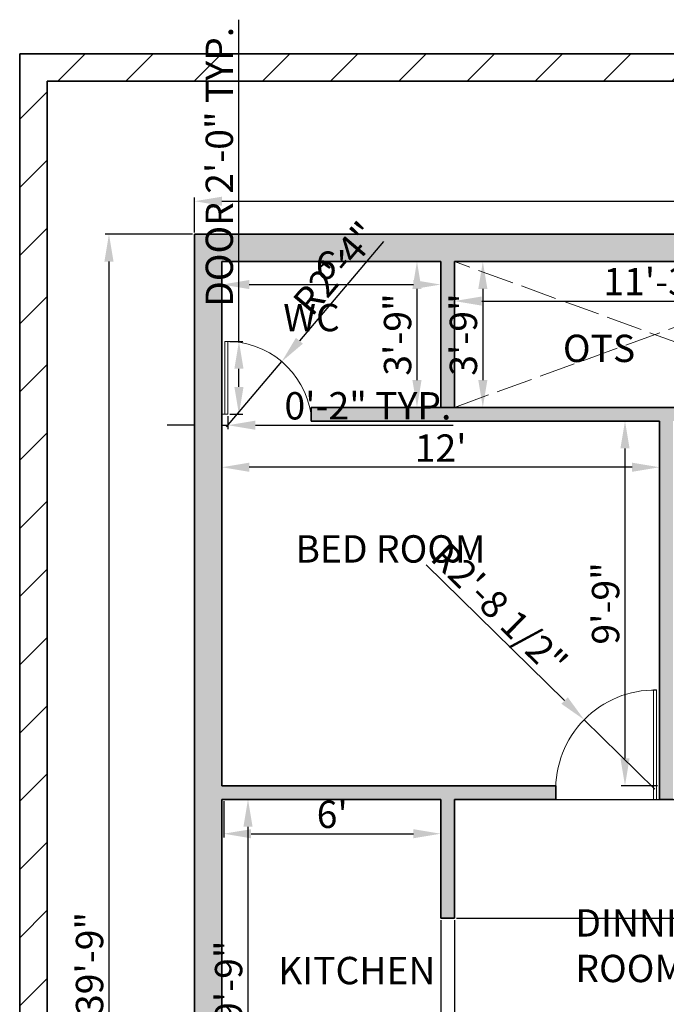
# Model space of a CAD drawing. Units: inches. Extents: x 1130698 to 1131150, y 432269 to 432875.
# Tile 2 of 3: x 1130698 to 1130911, y 432551 to 432875. Entities that reach past the tile are written whole.
import ezdxf

# ---------------------------------------------------------------- set-up
doc = ezdxf.new("R2010")
doc.units = ezdxf.units.IN
doc.linetypes.add('ACAD_ISO02W100', pattern=[15, 12, -3])
for name, color, linetype, lineweight in [('A-ANNO-DIMS', 2, 'Continuous', 18), ('A-ANNO-TTLB', 7, 'Continuous', 35), ('A-AREA-IDEN', 7, 'Continuous', 25), ('A-DOOR', 4, 'Continuous', 18), ('A-ROOF-OVHD', 8, 'ACAD_ISO02W100', 13), ('A-WALL', 7, 'Continuous', 35)]:
    doc.layers.add(name, color=color, linetype=linetype, lineweight=lineweight)
doc.layers.add('A-ANNO-TTLB-PATT', color=251, linetype='Continuous', lineweight=13, true_color=0x636466)
doc.layers.add('A-WALL-PATT', color=251, linetype='Continuous', lineweight=13, true_color=0x636466)
doc.styles.get("Standard").update_dxf_attribs({"font": 'arial.ttf'})
doc.dimstyles.new('ISO-25', dxfattribs={"dimtxt": 9, "dimasz": 9, "dimexe": 1.25, "dimexo": 0.625, "dimtad": 1, "dimdec": 1, "dimrnd": 9, "dimlunit": 3, "dimtxsty": 'Standard', "dimcen": 2.5, "dimadec": 0, "dimazin": 0, "dimtfac": 1, "dimtdec": 1, "dimtmove": 0, "dimatfit": 3, "dimfxl": 1, "dimarcsym": 0})

# ---------------------------------------------------------------- blocks, each defined once
blk = doc.blocks.new('*D1')
at = {"layer": 'A-ANNO-DIMS', "color": 0, "lineweight": -2, "transparency": 16777216}
for p, q in [((1130764.75, 432794.98), (1130764.75, 432786.8)), ((1130836.75, 432794.98), (1130836.75, 432786.8)), ((1130773.75, 432788.05), (1130827.75, 432788.05))]:
    blk.add_line(p, q, dxfattribs=at)
at = {"layer": 'A-ANNO-DIMS', "color": 0, "transparency": 16777216}
for points in [[(1130773.75, 432789.55), (1130773.75, 432786.55), (1130764.75, 432788.05)], [(1130827.75, 432789.55), (1130827.75, 432786.55), (1130836.75, 432788.05)]]:
    blk.add_solid(points, dxfattribs=at)
at = {"layer": 'Defpoints', "color": 0, "transparency": 16777216}
for p in [(1130764.75, 432795.61), (1130836.75, 432795.61), (1130836.75, 432788.05)]:
    blk.add_point(p, dxfattribs=at)
at = {"layer": 'A-ANNO-DIMS', "color": 0, "transparency": 16777216, "insert": (1130800.75, 432793.27), "char_height": 9, "attachment_point": 5}
blk.add_mtext("6'", dxfattribs=at)
blk = doc.blocks.new('*D2')
at = {"layer": 'A-ANNO-DIMS', "color": 0, "lineweight": -2, "transparency": 16777216}
for p, q in [((1130836.12, 432795.61), (1130827.69, 432795.61)), ((1130828.94, 432786.61), (1130828.94, 432756.61)), ((1130836.12, 432747.61), (1130827.69, 432747.61))]:
    blk.add_line(p, q, dxfattribs=at)
at = {"layer": 'A-ANNO-DIMS', "color": 0, "transparency": 16777216}
for points in [[(1130827.44, 432786.61), (1130830.44, 432786.61), (1130828.94, 432795.61)], [(1130827.44, 432756.61), (1130830.44, 432756.61), (1130828.94, 432747.61)]]:
    blk.add_solid(points, dxfattribs=at)
at = {"layer": 'Defpoints', "color": 0, "transparency": 16777216}
for p in [(1130836.75, 432795.61), (1130828.94, 432747.61), (1130836.75, 432747.61)]:
    blk.add_point(p, dxfattribs=at)
at = {"layer": 'A-ANNO-DIMS', "color": 0, "transparency": 16777216, "insert": (1130823.72, 432771.61), "char_height": 9, "attachment_point": 5, "rotation": 90}
blk.add_mtext('3\'-9"', dxfattribs=at)
blk = doc.blocks.new('*D3')
at = {"layer": 'A-ANNO-DIMS', "color": 0, "lineweight": -2, "transparency": 16777216}
for p, q in [((1130841.25, 432794.98), (1130841.25, 432781.37)), ((1130973.25, 432794.98), (1130973.25, 432781.37)), ((1130850.25, 432782.62), (1130964.25, 432782.62))]:
    blk.add_line(p, q, dxfattribs=at)
at = {"layer": 'A-ANNO-DIMS', "color": 0, "transparency": 16777216}
for points in [[(1130850.25, 432784.12), (1130850.25, 432781.12), (1130841.25, 432782.62)], [(1130964.25, 432784.12), (1130964.25, 432781.12), (1130973.25, 432782.62)]]:
    blk.add_solid(points, dxfattribs=at)
at = {"layer": 'Defpoints', "color": 0, "transparency": 16777216}
for p in [(1130841.25, 432795.61), (1130973.25, 432795.61), (1130973.25, 432782.62)]:
    blk.add_point(p, dxfattribs=at)
at = {"layer": 'A-ANNO-DIMS', "color": 0, "transparency": 16777216, "insert": (1130907.25, 432787.85), "char_height": 9, "attachment_point": 5}
blk.add_mtext('11\'-3"', dxfattribs=at)
blk = doc.blocks.new('*D4')
at = {"layer": 'A-ANNO-DIMS', "color": 0, "lineweight": -2, "transparency": 16777216}
for p, q in [((1130841.87, 432795.61), (1130851.87, 432795.61)), ((1130850.62, 432786.61), (1130850.62, 432756.61)), ((1130841.87, 432747.61), (1130851.87, 432747.61))]:
    blk.add_line(p, q, dxfattribs=at)
at = {"layer": 'A-ANNO-DIMS', "color": 0, "transparency": 16777216}
for points in [[(1130849.12, 432786.61), (1130852.12, 432786.61), (1130850.62, 432795.61)], [(1130849.12, 432756.61), (1130852.12, 432756.61), (1130850.62, 432747.61)]]:
    blk.add_solid(points, dxfattribs=at)
at = {"layer": 'Defpoints', "color": 0, "transparency": 16777216}
for p in [(1130841.25, 432795.61), (1130841.25, 432747.61), (1130850.62, 432747.61)]:
    blk.add_point(p, dxfattribs=at)
at = {"layer": 'A-ANNO-DIMS', "color": 0, "transparency": 16777216, "insert": (1130845.39, 432771.61), "char_height": 9, "attachment_point": 5, "rotation": 90}
blk.add_mtext('3\'-9"', dxfattribs=at)
blk = doc.blocks.new('*D7')
at = {"layer": 'A-ANNO-DIMS', "color": 0, "lineweight": -2, "transparency": 16777216}
for p, q in [((1130908.75, 432742.48), (1130908.75, 432726.67)), ((1130764.75, 432740.23), (1130764.75, 432726.67)), ((1130899.75, 432727.92), (1130773.75, 432727.92))]:
    blk.add_line(p, q, dxfattribs=at)
at = {"layer": 'A-ANNO-DIMS', "color": 0, "transparency": 16777216}
for points in [[(1130773.75, 432729.42), (1130773.75, 432726.42), (1130764.75, 432727.92)], [(1130899.75, 432729.42), (1130899.75, 432726.42), (1130908.75, 432727.92)]]:
    blk.add_solid(points, dxfattribs=at)
at = {"layer": 'Defpoints', "color": 0, "transparency": 16777216}
for p in [(1130908.75, 432743.11), (1130764.75, 432740.86), (1130764.75, 432727.92)]:
    blk.add_point(p, dxfattribs=at)
at = {"layer": 'A-ANNO-DIMS', "color": 0, "transparency": 16777216, "insert": (1130836.75, 432733.06), "char_height": 9, "attachment_point": 5}
blk.add_mtext("12'", dxfattribs=at)
blk = doc.blocks.new('*D8')
at = {"layer": 'A-ANNO-DIMS', "color": 0, "lineweight": -2, "transparency": 16777216}
for p, q in [((1130908.12, 432743.11), (1130896.15, 432743.11)), ((1130897.4, 432734.11), (1130897.4, 432632.11)), ((1130908.12, 432623.11), (1130896.15, 432623.11))]:
    blk.add_line(p, q, dxfattribs=at)
at = {"layer": 'A-ANNO-DIMS', "color": 0, "transparency": 16777216}
for points in [[(1130895.9, 432734.11), (1130898.9, 432734.11), (1130897.4, 432743.11)], [(1130895.9, 432632.11), (1130898.9, 432632.11), (1130897.4, 432623.11)]]:
    blk.add_solid(points, dxfattribs=at)
at = {"layer": 'Defpoints', "color": 0, "transparency": 16777216}
for p in [(1130908.75, 432743.11), (1130897.4, 432623.11), (1130908.75, 432623.11)]:
    blk.add_point(p, dxfattribs=at)
at = {"layer": 'A-ANNO-DIMS', "color": 0, "transparency": 16777216, "insert": (1130892.18, 432683.11), "char_height": 9, "attachment_point": 5, "rotation": 90}
blk.add_mtext('9\'-9"', dxfattribs=at)
blk = doc.blocks.new('*D13')
at = {"layer": 'A-ANNO-DIMS', "color": 0, "lineweight": -2, "transparency": 16777216}
for p, q in [((1130765.37, 432618.61), (1130774.58, 432618.61)), ((1130773.33, 432609.61), (1130773.33, 432507.61)), ((1130765.37, 432498.61), (1130774.58, 432498.61))]:
    blk.add_line(p, q, dxfattribs=at)
at = {"layer": 'A-ANNO-DIMS', "color": 0, "transparency": 16777216}
for points in [[(1130771.83, 432609.61), (1130774.83, 432609.61), (1130773.33, 432618.61)], [(1130771.83, 432507.61), (1130774.83, 432507.61), (1130773.33, 432498.61)]]:
    blk.add_solid(points, dxfattribs=at)
at = {"layer": 'Defpoints', "color": 0, "transparency": 16777216}
for p in [(1130764.75, 432618.61), (1130764.75, 432498.61), (1130773.33, 432498.61)]:
    blk.add_point(p, dxfattribs=at)
at = {"layer": 'A-ANNO-DIMS', "color": 0, "transparency": 16777216, "insert": (1130768.11, 432558.61), "char_height": 9, "attachment_point": 5, "rotation": 90}
blk.add_mtext('9\'-9"', dxfattribs=at)
blk = doc.blocks.new('*D14')
at = {"layer": 'A-ANNO-DIMS', "color": 0, "lineweight": -2, "transparency": 16777216}
for p, q in [((1130765.37, 432617.98), (1130765.37, 432606.05)), ((1130836.75, 432617.98), (1130836.75, 432606.05)), ((1130774.37, 432607.3), (1130827.75, 432607.3))]:
    blk.add_line(p, q, dxfattribs=at)
at = {"layer": 'A-ANNO-DIMS', "color": 0, "transparency": 16777216}
for points in [[(1130774.37, 432608.8), (1130774.37, 432605.8), (1130765.37, 432607.3)], [(1130827.75, 432608.8), (1130827.75, 432605.8), (1130836.75, 432607.3)]]:
    blk.add_solid(points, dxfattribs=at)
at = {"layer": 'Defpoints', "color": 0, "transparency": 16777216}
for p in [(1130765.37, 432618.61), (1130836.75, 432618.61), (1130836.75, 432607.3)]:
    blk.add_point(p, dxfattribs=at)
at = {"layer": 'A-ANNO-DIMS', "color": 0, "transparency": 16777216, "insert": (1130801.06, 432612.52), "char_height": 9, "attachment_point": 5}
blk.add_mtext("6'", dxfattribs=at)
blk = doc.blocks.new('*D20')
at = {"layer": 'A-ANNO-DIMS', "color": 0, "lineweight": -2, "transparency": 16777216}
for p, q in [((1130755.75, 432805.23), (1130755.75, 432816.73)), ((1131115.75, 432805.23), (1131115.75, 432816.73)), ((1130764.75, 432815.48), (1131106.75, 432815.48))]:
    blk.add_line(p, q, dxfattribs=at)
at = {"layer": 'A-ANNO-DIMS', "color": 0, "transparency": 16777216}
for points in [[(1130764.75, 432816.98), (1130764.75, 432813.98), (1130755.75, 432815.48)], [(1131106.75, 432816.98), (1131106.75, 432813.98), (1131115.75, 432815.48)]]:
    blk.add_solid(points, dxfattribs=at)
at = {"layer": 'Defpoints', "color": 0, "transparency": 16777216}
for p in [(1131115.75, 432815.48), (1130755.75, 432804.61), (1131115.75, 432804.61)]:
    blk.add_point(p, dxfattribs=at)
at = {"layer": 'A-ANNO-DIMS', "color": 0, "transparency": 16777216, "insert": (1130935.75, 432820.71), "char_height": 9, "attachment_point": 5}
blk.add_mtext("30'", dxfattribs=at)
blk = doc.blocks.new('*D21')
at = {"layer": 'A-ANNO-DIMS', "color": 0, "lineweight": -2, "transparency": 16777216}
for p, q in [((1130755.12, 432804.61), (1130726.33, 432804.61)), ((1130727.58, 432795.61), (1130727.58, 432333.61)), ((1130755.12, 432324.61), (1130726.33, 432324.61))]:
    blk.add_line(p, q, dxfattribs=at)
at = {"layer": 'A-ANNO-DIMS', "color": 0, "transparency": 16777216}
for points in [[(1130726.08, 432795.61), (1130729.08, 432795.61), (1130727.58, 432804.61)], [(1130726.08, 432333.61), (1130729.08, 432333.61), (1130727.58, 432324.61)]]:
    blk.add_solid(points, dxfattribs=at)
at = {"layer": 'Defpoints', "color": 0, "transparency": 16777216}
for p in [(1130755.75, 432804.61), (1130727.58, 432324.61), (1130755.75, 432324.61)]:
    blk.add_point(p, dxfattribs=at)
at = {"layer": 'A-ANNO-DIMS', "color": 0, "transparency": 16777216, "insert": (1130722.35, 432564.61), "char_height": 9, "attachment_point": 5, "rotation": 90}
blk.add_mtext('39\'-9"', dxfattribs=at)
blk = doc.blocks.new('DOOR-LEAF-36IN')
for p, q in [((0, 2), (0, 1)), ((0, 1), (36, 1)), ((0, 0), (0, 1)), ((36, 1), (36, 0)), ((36, 0), (0, 0))]:
    blk.add_line(p, q)
blk = doc.blocks.new('DOOR-LEAF-24IN')
for p, q in [((1, 0), (1, 24)), ((1, 24), (2, 24)), ((2, 24), (2, 0)), ((0, 0), (1, 0)), ((2, 0), (1, 0))]:
    blk.add_line(p, q)
blk = doc.blocks.new('*D30')
at = {"layer": 'A-ANNO-DIMS', "color": 0, "lineweight": -2, "transparency": 16777216}
for p, q in [((1130770.35, 432769.36), (1130770.35, 432875.23)), ((1130767.37, 432769.36), (1130771.6, 432769.36)), ((1130770.35, 432754.36), (1130770.35, 432760.36)), ((1130767.37, 432745.36), (1130771.6, 432745.36))]:
    blk.add_line(p, q, dxfattribs=at)
at = {"layer": 'A-ANNO-DIMS', "color": 0, "transparency": 16777216}
for points in [[(1130768.85, 432760.36), (1130771.85, 432760.36), (1130770.35, 432769.36)], [(1130768.85, 432754.36), (1130771.85, 432754.36), (1130770.35, 432745.36)]]:
    blk.add_solid(points, dxfattribs=at)
at = {"layer": 'Defpoints', "color": 0, "transparency": 16777216}
for p in [(1130766.75, 432769.36), (1130770.35, 432769.36), (1130766.75, 432745.36)]:
    blk.add_point(p, dxfattribs=at)
at = {"layer": 'A-ANNO-DIMS', "color": 0, "transparency": 16777216, "insert": (1130765.06, 432826.79), "char_height": 9, "attachment_point": 5, "rotation": 90}
blk.add_mtext('DOOR 2\'-0" TYP.', dxfattribs=at)
blk = doc.blocks.new('*D31')
at = {"layer": 'A-ANNO-DIMS', "color": 0, "lineweight": -2, "transparency": 16777216}
for p, q in [((1130755.75, 432741.76), (1130746.75, 432741.76)), ((1130764.75, 432744.73), (1130764.75, 432740.51)), ((1130764.75, 432741.76), (1130766.75, 432741.76)), ((1130766.75, 432744.73), (1130766.75, 432740.51)), ((1130775.75, 432741.76), (1130840.86, 432741.76))]:
    blk.add_line(p, q, dxfattribs=at)
at = {"layer": 'A-ANNO-DIMS', "color": 0, "transparency": 16777216}
for points in [[(1130755.75, 432743.26), (1130755.75, 432740.26), (1130764.75, 432741.76)], [(1130775.75, 432743.26), (1130775.75, 432740.26), (1130766.75, 432741.76)]]:
    blk.add_solid(points, dxfattribs=at)
at = {"layer": 'Defpoints', "color": 0, "transparency": 16777216}
for p in [(1130764.75, 432745.36), (1130766.75, 432745.36), (1130766.75, 432741.76)]:
    blk.add_point(p, dxfattribs=at)
at = {"layer": 'A-ANNO-DIMS', "color": 0, "transparency": 16777216, "insert": (1130812.8, 432746.98), "char_height": 9, "attachment_point": 5}
blk.add_mtext('0\'-2" TYP.', dxfattribs=at)
blk = doc.blocks.new('*D36')
at = {"layer": 'A-ANNO-DIMS', "color": 0, "lineweight": -2, "transparency": 16777216}
for p, q in [((1130841.96, 432579.47), (1131143.2, 432579.47)), ((1131141.95, 432570.47), (1131141.95, 432554.94)), ((1130842.05, 432545.94), (1131143.2, 432545.94)), ((1131141.95, 432545.94), (1131141.95, 432490.64))]:
    blk.add_line(p, q, dxfattribs=at)
at = {"layer": 'A-ANNO-DIMS', "color": 0, "transparency": 16777216}
for points in [[(1131140.45, 432570.47), (1131143.45, 432570.47), (1131141.95, 432579.47)], [(1131140.45, 432554.94), (1131143.45, 432554.94), (1131141.95, 432545.94)]]:
    blk.add_solid(points, dxfattribs=at)
at = {"layer": 'Defpoints', "color": 0, "transparency": 16777216}
for p in [(1130841.34, 432579.47), (1130841.42, 432545.94), (1131141.95, 432545.94)]:
    blk.add_point(p, dxfattribs=at)
at = {"layer": 'A-ANNO-DIMS', "color": 0, "transparency": 16777216, "insert": (1131136.67, 432513.79), "char_height": 9, "attachment_point": 5, "rotation": 90}
blk.add_mtext('2\'-9 1/2"', dxfattribs=at)
blk = doc.blocks.new('*D37')
at = {"layer": 'A-ANNO-DIMS', "color": 0, "lineweight": -2, "transparency": 16777216}
for p, q in [((1130841.87, 432618.61), (1131143.2, 432618.61)), ((1131141.95, 432609.61), (1131141.95, 432588.47)), ((1130841.96, 432579.47), (1131143.2, 432579.47))]:
    blk.add_line(p, q, dxfattribs=at)
at = {"layer": 'A-ANNO-DIMS', "color": 0, "transparency": 16777216}
for points in [[(1131140.45, 432609.61), (1131143.45, 432609.61), (1131141.95, 432618.61)], [(1131140.45, 432588.47), (1131143.45, 432588.47), (1131141.95, 432579.47)]]:
    blk.add_solid(points, dxfattribs=at)
at = {"layer": 'Defpoints', "color": 0, "transparency": 16777216}
for p in [(1130841.25, 432618.61), (1130841.34, 432579.47), (1131141.95, 432579.47)]:
    blk.add_point(p, dxfattribs=at)
at = {"layer": 'A-ANNO-DIMS', "color": 0, "transparency": 16777216, "insert": (1131136.72, 432599.04), "char_height": 9, "attachment_point": 5, "rotation": 90}
blk.add_mtext('3\'-3"', dxfattribs=at)
blk = doc.blocks.new('*D41')
at = {"layer": 'A-ANNO-DIMS', "color": 0, "lineweight": -2, "transparency": 16777216}
for p, q in [((1130836.75, 432578.84), (1130836.75, 432297.16)), ((1130841.34, 432578.84), (1130841.34, 432297.16)), ((1130827.75, 432298.41), (1130818.75, 432298.41)), ((1130836.75, 432298.41), (1130841.34, 432298.41)), ((1130850.34, 432298.41), (1130905.49, 432298.41))]:
    blk.add_line(p, q, dxfattribs=at)
at = {"layer": 'A-ANNO-DIMS', "color": 0, "transparency": 16777216}
for points in [[(1130827.75, 432299.91), (1130827.75, 432296.91), (1130836.75, 432298.41)], [(1130850.34, 432299.91), (1130850.34, 432296.91), (1130841.34, 432298.41)]]:
    blk.add_solid(points, dxfattribs=at)
at = {"layer": 'Defpoints', "color": 0, "transparency": 16777216}
for p in [(1130836.75, 432579.47), (1130841.34, 432579.47), (1130841.34, 432298.41)]:
    blk.add_point(p, dxfattribs=at)
at = {"layer": 'A-ANNO-DIMS', "color": 0, "transparency": 16777216, "insert": (1130882.41, 432303.68), "char_height": 9, "attachment_point": 5}
blk.add_mtext('0\'-4 1/2"', dxfattribs=at)
blk = doc.blocks.new('*D44')
at = {"layer": 'A-ANNO-DIMS', "color": 0, "lineweight": -2, "transparency": 16777216}
for p, q in [((1130832.02, 432695.79), (1130877.53, 432651.13)), ((1130907.25, 432621.97), (1130883.95, 432644.83))]:
    blk.add_line(p, q, dxfattribs=at)
at = {"layer": 'A-ANNO-DIMS', "color": 0, "transparency": 16777216}
blk.add_solid([(1130878.58, 432652.2), (1130876.48, 432650.06), (1130883.95, 432644.83)], dxfattribs=at)
at = {"layer": 'Defpoints', "color": 0, "transparency": 16777216}
for p in [(1130883.95, 432644.83), (1130907.25, 432621.97)]:
    blk.add_point(p, dxfattribs=at)
at = {"layer": 'A-ANNO-DIMS', "color": 0, "transparency": 16777216, "insert": (1130855.26, 432680.38), "char_height": 9, "attachment_point": 5, "rotation": 315.5434}
blk.add_mtext('R2\'-8 1/2"', dxfattribs=at)
blk = doc.blocks.new('*D46')
at = {"layer": 'A-ANNO-DIMS', "color": 0, "lineweight": -2, "transparency": 16777216}
for p, q in [((1130817.9, 432802.22), (1130790.25, 432769.56)), ((1130766.25, 432741.21), (1130784.44, 432762.69))]:
    blk.add_line(p, q, dxfattribs=at)
at = {"layer": 'A-ANNO-DIMS', "color": 0, "transparency": 16777216}
blk.add_solid([(1130789.11, 432770.53), (1130791.4, 432768.59), (1130784.44, 432762.69)], dxfattribs=at)
at = {"layer": 'Defpoints', "color": 0, "transparency": 16777216}
for p in [(1130784.44, 432762.69), (1130766.25, 432741.21)]:
    blk.add_point(p, dxfattribs=at)
at = {"layer": 'A-ANNO-DIMS', "color": 0, "transparency": 16777216, "insert": (1130803.06, 432792.65), "char_height": 9, "attachment_point": 5, "rotation": 49.7462}
blk.add_mtext('R2\'-4"', dxfattribs=at)

msp = doc.modelspace()

# ---------------------------------------------------------------- hatches: boundary and pattern name
at = {"layer": 'A-ANNO-TTLB-PATT'}
h = msp.add_hatch(dxfattribs=at)
h.set_pattern_fill('ANSI31', color=256, scale=5)
h.paths.add_polyline_path([(1131144.8, 432864.01), (1130698.2, 432864.01), (1130698.2, 432276.41), (1131144.8, 432276.41)])
h.paths.add_polyline_path([(1130707.2, 432855.01), (1131135.8, 432855.01), (1131135.8, 432285.41), (1130707.2, 432285.41)], flags=16)
h.paths.add_polyline_path([(1130755.75, 432804.61), (1131115.75, 432804.61), (1131115.75, 432324.61), (1130908.75, 432324.61), (1130908.75, 432333.61), (1131106.75, 432333.61), (1131106.75, 432494.61), (1131076.75, 432494.61), (1131076.75, 432370.11), (1130908.75, 432370.11), (1130908.75, 432352.4), (1130764.75, 432352.4), (1130764.75, 432333.61), (1130764.75, 432324.61), (1130755.75, 432324.61)], flags=0)
h.paths.add_polyline_path([(1130764.75, 432795.61), (1130836.75, 432795.61), (1130836.75, 432747.61), (1130841.25, 432747.61), (1130841.25, 432795.61), (1130973.25, 432795.61), (1130973.25, 432747.61), (1130977.75, 432747.61), (1130977.75, 432795.61), (1130986.75, 432795.61), (1131106.75, 432795.61), (1131106.75, 432499.11), (1130973.25, 432499.11), (1130973.25, 432498.61), (1130959.44, 432498.61), (1130959.45, 432494.57), (1130973.25, 432494.61), (1131072.25, 432494.61), (1131072.25, 432374.61), (1130913.25, 432374.61), (1130913.25, 432379.9), (1130911, 432379.9), (1130911, 432380.9), (1130911, 432381.9), (1130941, 432381.9, 0.411251), (1130913.25, 432408.94), (1130908.75, 432408.94), (1130908.75, 432498.61), (1130907.75, 432498.61), (1130907.75, 432468.61, -0.386197), (1130873.7, 432498.61), (1130873.7, 432494.37), (1130841.54, 432494.37), (1130841.42, 432545.94), (1130836.75, 432545.94), (1130836.75, 432498.61), (1130764.75, 432498.61), (1130764.75, 432618.61), (1130836.75, 432618.61), (1130836.75, 432579.47), (1130841.34, 432579.47), (1130841.25, 432618.61), (1130874.63, 432618.61), (1130874.63, 432620.86, -0.017137), (1130874.63, 432623.09), (1130874.63, 432623.11), (1130764.75, 432623.11), (1130764.75, 432738.61), (1130764.75, 432743.11), (1130764.75, 432747.61)], flags=0)
h.paths.add_polyline_path([(1130765.75, 432769.36, -0.376584), (1130794.09, 432745.36), (1130794.09, 432743.11), (1130908.75, 432743.11), (1130908.75, 432618.61), (1130913.25, 432618.61), (1130913.25, 432743.11), (1130973.25, 432743.11), (1130973.25, 432664.11), (1130938.73, 432664.11), (1130938.73, 432659.61), (1130977.75, 432659.61, -0.392039), (1131009.25, 432624.61), (1130973.25, 432624.61), (1130973.25, 432623.61), (1130973.25, 432619.11), (1130973.25, 432618.11), (1131009.25, 432618.11, -0.432961), (1130975.5, 432585.44), (1130977.75, 432585.44), (1130977.75, 432585.41, 0.403315), (1131009.25, 432617.11), (1130973.25, 432617.11), (1130973.25, 432618.11), (1130973.25, 432619.11), (1130973.25, 432623.61), (1130973.25, 432624.61), (1130973.25, 432625.61), (1131009.25, 432625.61, 0.383736), (1130977.75, 432659.61), (1130938.73, 432659.61, 0.405522), (1130915.25, 432683.38), (1130915.25, 432659.38), (1130914.25, 432659.38), (1130913.25, 432659.38), (1130913.25, 432618.61), (1130908.75, 432618.61), (1130907.75, 432618.61), (1130906.75, 432618.61), (1130906.75, 432654.61), (1130907.75, 432654.61), (1130907.75, 432618.61), (1130908.75, 432618.61), (1130908.75, 432743.11), (1130794.09, 432743.11), (1130794.09, 432745.36, 0.366478), (1130766.75, 432769.36), (1130766.75, 432745.36), (1130765.75, 432745.36)], flags=0)
h.paths.add_polyline_path([(1130782.75, 432476.15), (1130836.75, 432476.19), (1130836.75, 432458.28), (1130800.75, 432458.19), (1130800.75, 432398.19), (1130812.75, 432398.22), (1130812.75, 432362.22), (1130765.06, 432362.11), (1130782.9, 432380.15)], flags=0)
h.paths.add_polyline_path([(1130794.59, 432383.39), (1130800.75, 432380.15), (1130794.59, 432377.08)], flags=0)
h.paths.add_polyline_path([(1130793.86, 432783.91), (1130807.75, 432783.91), (1130807.75, 432802.46), (1130793.86, 432802.46)], flags=8)
h.paths.add_polyline_path([(1130833.23, 432764.87), (1130833.23, 432778.77), (1130814.69, 432778.77), (1130814.69, 432764.87)], flags=8)
h.paths.add_polyline_path([(1130888.59, 432778.49), (1130925.12, 432778.49), (1130925.12, 432797.04), (1130888.59, 432797.04)], flags=8)
h.paths.add_polyline_path([(1130854.91, 432764.87), (1130854.91, 432778.77), (1130836.36, 432778.77), (1130836.36, 432764.87)], flags=8)
h.paths.add_polyline_path([(1131023.59, 432772.28), (1131060.12, 432772.28), (1131060.12, 432790.83), (1131023.59, 432790.83)], flags=8)
h.paths.add_polyline_path([(1130825.91, 432723.63), (1130846.8, 432723.63), (1130846.8, 432742.18), (1130825.91, 432742.18)], flags=8)
h.paths.add_polyline_path([(1130901.54, 432668.37), (1130901.54, 432697.91), (1130882.99, 432697.91), (1130882.99, 432668.37)], flags=8)
h.paths.add_polyline_path([(1130928.51, 432726.62), (1130958.05, 432726.62), (1130958.05, 432745.17), (1130928.51, 432745.17)], flags=8)
h.paths.add_polyline_path([(1130972.51, 432688.9), (1130972.51, 432718.43), (1130953.97, 432718.43), (1130953.97, 432688.9)], flags=8)
h.paths.add_polyline_path([(1130925.33, 432811.35), (1130946.22, 432811.35), (1130946.22, 432829.9), (1130925.33, 432829.9)], flags=8)
h.paths.add_polyline_path([(1130731.71, 432554.38), (1130731.71, 432575.26), (1130713.17, 432575.26), (1130713.17, 432554.38)], flags=8)
h.paths.add_polyline_path([(1130755.82, 432293.19), (1130947.18, 432293.19), (1130947.18, 432317.92), (1130755.82, 432317.92)], flags=8)
h.paths.add_polyline_path([(1130779.57, 432338.43), (1130829.48, 432338.43), (1130829.48, 432356.98), (1130779.57, 432356.98)], flags=8)
h.paths.add_polyline_path([(1130969.67, 432346.11), (1131010.5, 432346.11), (1131010.5, 432364.66), (1130969.67, 432364.66)], flags=8)
h.paths.add_polyline_path([(1130950.99, 432437.85), (1131016.28, 432437.85), (1131016.28, 432471.55), (1130950.99, 432471.55)], flags=8)
h.paths.add_polyline_path([(1130780.08, 432552.69), (1130839.77, 432552.69), (1130839.77, 432571.24), (1130780.08, 432571.24)], flags=8)
h.paths.add_polyline_path([(1130996.81, 432568.37), (1131080.25, 432568.37), (1131080.25, 432586.92), (1130996.81, 432586.92)], flags=8)
h.paths.add_polyline_path([(1130877.83, 432553.22), (1130935.44, 432553.22), (1130935.44, 432586.93), (1130877.83, 432586.93)], flags=8)
h.paths.add_polyline_path([(1130919.84, 432705.86), (1130945.29, 432705.86), (1130945.29, 432724.41), (1130919.84, 432724.41)], flags=8)
h.paths.add_polyline_path([(1131004.1, 432697.07), (1131077.07, 432697.07), (1131077.07, 432730.77), (1131004.1, 432730.77)], flags=8)
h.paths.add_polyline_path([(1130782.53, 432767.61), (1130807.98, 432767.61), (1130807.98, 432786.15), (1130782.53, 432786.15)], flags=8)
h.paths.add_polyline_path([(1130874.11, 432757.47), (1130904.45, 432757.47), (1130904.45, 432776.02), (1130874.11, 432776.02)], flags=8)
h.paths.add_polyline_path([(1130785.78, 432691.47), (1130858.74, 432691.47), (1130858.74, 432710.01), (1130785.78, 432710.01)], flags=8)
at = {"layer": 'A-WALL-PATT'}
h = msp.add_hatch(color=256, dxfattribs=at)
h.dxf.hatch_style = 1
h.paths.add_polyline_path([(1130764.75, 432738.61), (1130764.75, 432743.11), (1130764.75, 432747.61), (1130764.75, 432795.61), (1130836.75, 432795.61), (1130836.75, 432747.61), (1130841.25, 432747.61), (1130841.25, 432795.61), (1130973.25, 432795.61), (1130973.25, 432747.61), (1130977.75, 432747.61), (1130977.75, 432795.61), (1130986.75, 432795.61), (1131106.75, 432795.61), (1131106.75, 432499.11), (1131106.75, 432494.61), (1131115.75, 432494.61), (1131115.75, 432804.61), (1130755.75, 432804.61), (1130755.75, 432494.37), (1130841.54, 432494.37), (1130841.42, 432545.94), (1130836.75, 432545.94), (1130836.75, 432498.61), (1130764.75, 432498.61), (1130764.75, 432618.61), (1130836.75, 432618.61), (1130836.75, 432579.47), (1130841.34, 432579.47), (1130841.25, 432618.61), (1130874.63, 432618.61), (1130874.63, 432623.11), (1130764.75, 432623.11)])
h.paths.add_polyline_path([(1131106.75, 432623.61), (1130973.25, 432623.61), (1130973.25, 432619.11), (1131106.75, 432619.11)], flags=17)
h.paths.add_polyline_path([(1130913.25, 432743.11), (1130973.25, 432743.11), (1130973.25, 432664.11), (1130938.73, 432664.11), (1130938.73, 432659.61), (1130977.75, 432659.61), (1130977.75, 432743.11), (1130977.75, 432747.61), (1130973.25, 432747.61), (1130794.09, 432747.61), (1130794.09, 432743.11), (1130908.75, 432743.11), (1130908.75, 432618.61), (1130913.25, 432618.61)], flags=17)
h.paths.add_polyline_path([(1131076.75, 432499.11), (1130973.25, 432499.11), (1130973.25, 432498.61), (1130959.44, 432498.61), (1130959.45, 432494.57), (1130973.25, 432494.61), (1131072.25, 432494.61), (1131072.25, 432374.61), (1130913.25, 432374.61), (1130913.25, 432379.9), (1130908.75, 432379.9), (1130908.75, 432370.11), (1131076.75, 432370.11)])
h.paths.add_polyline_path([(1130977.75, 432585.41, -0.017472), (1130975.5, 432585.44), (1130973.25, 432585.44), (1130973.25, 432499.11), (1130977.75, 432499.11)], flags=17)
h.paths.add_polyline_path([(1130873.7, 432498.61), (1130841.53, 432498.61), (1130841.54, 432494.37), (1130873.7, 432494.37)], flags=17)
h.paths.add_polyline_path([(1130913.25, 432494.46), (1130927.62, 432494.5), (1130927.61, 432498.61), (1130908.75, 432498.61), (1130908.75, 432408.94), (1130913.25, 432408.94)])

# ---------------------------------------------------------------- linework, layer by layer
at = {"layer": 'A-ANNO-TTLB'}
for points in [[(1130698.2, 432864.01), (1131144.8, 432864.01), (1131144.8, 432276.41), (1130698.2, 432276.41)], [(1130707.2, 432855.01), (1131135.8, 432855.01), (1131135.8, 432285.41), (1130707.2, 432285.41)]]:
    msp.add_lwpolyline(points, close=True, dxfattribs=at)
at = {"layer": 'A-DOOR'}
for centre, radius, start, end in [((1130766.25, 432741.21), 28.15, 8.4754, 91.0176), ((1130907.25, 432621.97), 32.64, 89.1222, 181.9635)]:
    msp.add_arc(centre, radius, start, end, dxfattribs=at)
at = {"layer": 'A-ROOF-OVHD'}
for p, q in [((1130973.25, 432747.61), (1130841.25, 432795.61)), ((1130841.25, 432747.61), (1130973.25, 432795.61))]:
    msp.add_line(p, q, dxfattribs=at)
at = {"layer": 'A-WALL'}
for p, q in [((1131115.75, 432804.61), (1130755.75, 432804.61)), ((1130755.75, 432804.61), (1130755.75, 432324.61)), ((1130764.75, 432795.61), (1130764.75, 432747.61)), ((1130836.75, 432795.61), (1130764.75, 432795.61)), ((1130836.75, 432795.61), (1130836.75, 432747.61)), ((1130841.25, 432795.61), (1130841.25, 432747.61)), ((1130973.25, 432795.61), (1130841.25, 432795.61)), ((1130764.75, 432747.61), (1130764.75, 432743.11)), ((1130977.75, 432747.61), (1130794.09, 432747.61)), ((1130794.09, 432747.61), (1130794.09, 432743.11)), ((1130764.75, 432743.11), (1130764.75, 432738.61)), ((1130908.75, 432743.11), (1130794.09, 432743.11)), ((1130908.75, 432743.11), (1130908.75, 432618.61)), ((1130764.75, 432738.61), (1130764.75, 432623.11)), ((1130874.63, 432623.11), (1130764.75, 432623.11)), ((1130874.63, 432623.11), (1130874.63, 432618.61)), ((1130764.75, 432618.61), (1130764.75, 432498.61)), ((1130836.75, 432618.61), (1130764.75, 432618.61)), ((1130836.75, 432618.61), (1130836.75, 432579.47)), ((1130874.63, 432618.61), (1130841.25, 432618.61)), ((1130841.25, 432618.61), (1130841.34, 432579.47)), ((1130913.25, 432618.61), (1130908.75, 432618.61)), ((1130841.34, 432579.47), (1130836.75, 432579.47))]:
    msp.add_line(p, q, dxfattribs=at)

# ---------------------------------------------------------------- block references
at = {"layer": 'A-DOOR'}
msp.add_blockref('DOOR-LEAF-24IN', (1130764.75, 432745.36), dxfattribs=at)
at = {"layer": 'A-DOOR', "extrusion": (0, 0, -1), "zscale": -1, "rotation": 90.0000000007512}
msp.add_blockref('DOOR-LEAF-36IN', (-1130906.75, 432618.61), dxfattribs=at)

# ---------------------------------------------------------------- texts
at = {"layer": 'A-AREA-IDEN', "char_height": 9, "attachment_point": 1}
for s, insert in [('WC', (1130784.93, 432781.68)), ('OTS', (1130876.97, 432771.55)), ('BED ROOM', (1130788.95, 432705.54)), ('DINNING\\PROOM', (1130881.07, 432582.45)), ('KITCHEN', (1130783.25, 432566.76))]:
    msp.add_mtext_dynamic_manual_height_columns(s, width=84.4356, gutter_width=12.5, heights=[0], dxfattribs=dict(at, insert=insert))

# ---------------------------------------------------------------- dimensions: what is measured, and where the dimension line sits
at = {"layer": 'A-ANNO-DIMS'}
dim = msp.add_linear_dim(base=(1130770.35, 432769.36), p1=(1130766.75, 432745.36), p2=(1130766.75, 432769.36), angle=90, text='DOOR <> TYP.', dimstyle='ISO-25', override={"dimdec": 1, "dimlfac": 1, "dimrnd": 0, "dimzin": 1, "dimdsep": 46, "dimlunit": 4, "dimfrac": 2}, dxfattribs=at)
dim.commit()
dim.dimension.update_dxf_attribs({"geometry": '*D30', "text_midpoint": (1130765.06, 432826.79)})
for base, p1, p2, override, picture, middle in [((1131115.75, 432815.48), (1130755.75, 432804.61), (1131115.75, 432804.61), {"dimclrd": 0, "dimclre": 0, "dimclrt": 0}, '*D20', (1130935.75, 432820.71)), ((1130836.75, 432788.05), (1130764.75, 432795.61), (1130836.75, 432795.61), {"dimclrd": 0, "dimclre": 0, "dimclrt": 0}, '*D1', (1130800.75, 432793.27)), ((1130973.25, 432782.62), (1130841.25, 432795.61), (1130973.25, 432795.61), {"dimclrd": 0, "dimclre": 0, "dimclrt": 0}, '*D3', (1130907.25, 432787.85)), ((1130764.75, 432727.92), (1130908.75, 432743.11), (1130764.75, 432740.86), {"dimclrd": 0, "dimclre": 0, "dimclrt": 0}, '*D7', (1130836.75, 432733.06)), ((1130836.75, 432607.3), (1130765.37, 432618.61), (1130836.75, 432618.61), {"dimclrd": 0, "dimclre": 0, "dimclrt": 0}, '*D14', (1130801.06, 432612.52)), ((1130841.34, 432298.41), (1130836.75, 432579.47), (1130841.34, 432579.47), {"dimdec": 1, "dimlfac": 1, "dimrnd": 0, "dimzin": 1, "dimdsep": 46, "dimlunit": 4, "dimfrac": 2}, '*D41', (1130882.41, 432303.68))]:
    dim = msp.add_linear_dim(base=base, p1=p1, p2=p2, dimstyle='ISO-25', override=override, dxfattribs=at)
    dim.commit()
    dim.dimension.update_dxf_attribs({"geometry": picture, "text_midpoint": middle})
for center, mpoint, picture, middle in [((1130766.2458, 432741.2063), (1130784.4381, 432762.6931), '*D46', (1130803.0601, 432792.6472)), ((1130907.25, 432621.97), (1130883.95, 432644.83), '*D44', (1130855.26, 432680.38))]:
    dim = msp.add_radius_dim(center=center, mpoint=mpoint, dimstyle='ISO-25', override={"dimdec": 1, "dimlfac": 1, "dimrnd": 0, "dimzin": 1, "dimdsep": 46, "dimlunit": 4, "dimfrac": 2}, dxfattribs=at)
    dim.commit()
    dim.dimension.update_dxf_attribs({"geometry": picture, "text_midpoint": middle})
for base, p1, p2, override, picture, middle in [((1130727.58, 432324.61), (1130755.75, 432804.61), (1130755.75, 432324.61), {"dimclrd": 0, "dimclre": 0, "dimclrt": 0}, '*D21', (1130722.35, 432564.61)), ((1130828.94, 432747.61), (1130836.75, 432795.61), (1130836.75, 432747.61), {"dimclrd": 0, "dimclre": 0, "dimclrt": 0}, '*D2', (1130823.72, 432771.61)), ((1130850.62, 432747.61), (1130841.25, 432795.61), (1130841.25, 432747.61), {"dimclrd": 0, "dimclre": 0, "dimclrt": 0}, '*D4', (1130845.39, 432771.61)), ((1130897.4, 432623.11), (1130908.75, 432743.11), (1130908.75, 432623.11), {"dimclrd": 0, "dimclre": 0, "dimclrt": 0}, '*D8', (1130892.18, 432683.11)), ((1130773.33, 432498.61), (1130764.75, 432618.61), (1130764.75, 432498.61), {"dimclrd": 0, "dimclre": 0, "dimclrt": 0}, '*D13', (1130768.11, 432558.61)), ((1131141.95, 432579.47), (1130841.25, 432618.61), (1130841.34, 432579.47), {"dimdec": 1, "dimlfac": 1, "dimrnd": 0, "dimzin": 1, "dimdsep": 46, "dimlunit": 4, "dimfrac": 2}, '*D37', (1131136.72, 432599.04)), ((1131141.95, 432545.94), (1130841.34, 432579.47), (1130841.42, 432545.94), {"dimdec": 1, "dimlfac": 1, "dimrnd": 0, "dimzin": 1, "dimdsep": 46, "dimlunit": 4, "dimfrac": 2}, '*D36', (1131136.67, 432513.79))]:
    dim = msp.add_linear_dim(base=base, p1=p1, p2=p2, angle=90, dimstyle='ISO-25', override=override, dxfattribs=at)
    dim.commit()
    dim.dimension.update_dxf_attribs({"geometry": picture, "text_midpoint": middle})
dim = msp.add_linear_dim(base=(1130766.75, 432741.76), p1=(1130764.75, 432745.36), p2=(1130766.75, 432745.36), text='<> TYP.', dimstyle='ISO-25', override={"dimdec": 1, "dimlfac": 1, "dimrnd": 0, "dimzin": 1, "dimdsep": 46, "dimlunit": 4, "dimfrac": 2}, dxfattribs=at)
dim.commit()
dim.dimension.update_dxf_attribs({"geometry": '*D31', "text_midpoint": (1130812.8, 432746.98)})

doc.saveas('drawing.dxf')
